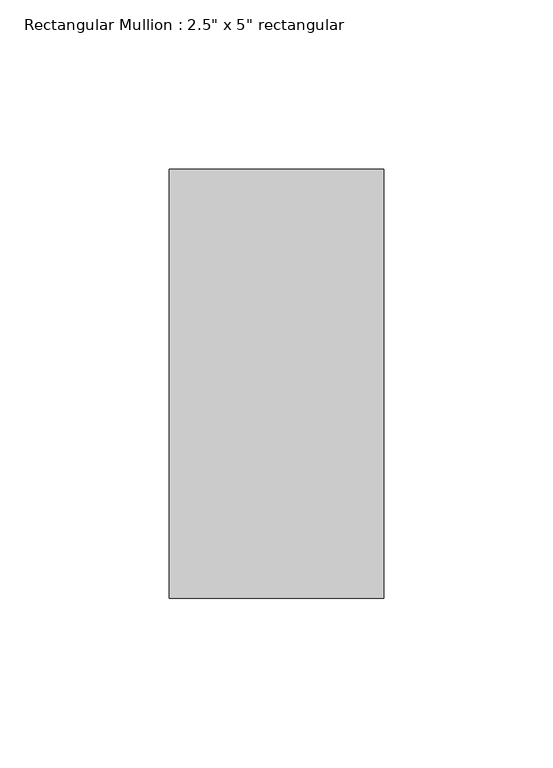
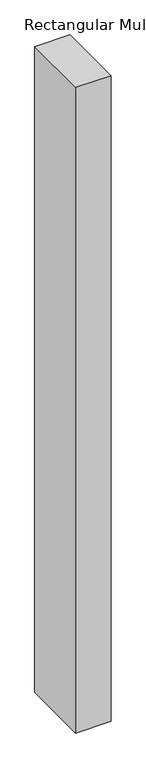
"""IFC4 building model written with IfcOpenShell, lengths in millimetres: member geometry."""

from ifc_helpers import new_model, si_unit, frame, origin, place, context, project, spatial, polyline, outline, extrude, source, transform, mapped, element, save


def member_d722639b(model_context):
    return source(origin(), model_context, "Body", "SweptSolid", [
        extrude(outline(polyline([(0.0, 63.5), (0.0, -63.5), (-63.5, -63.5), (-63.5, 63.5), (0.0, 63.5)])), frame((0.0, 0.0, -1224.7874211), z_axis=(0.0, 0.0, 1.0), x_axis=(1.0, 0.0, 0.0)), (0.0, 0.0, 1.0), 1224.7874211),
    ])


if __name__ == "__main__":
    model = new_model("IFC4")
    model_context = context("Model", 3, world=origin())
    ifc_project = project(units=[si_unit("LENGTHUNIT", "METRE", prefix="MILLI")], contexts=[model_context])
    site = spatial("IfcSite", under=ifc_project)
    building = spatial("IfcBuilding", under=site)
    placement = place(None, origin())
    member_shape = member_d722639b(model_context)
    element("IfcMember", 1, ObjectType="Rectangular Mullion : 2.5\" x 5\" rectangular", at=placement, inside=building, context=model_context, shape_type="MappedRepresentation", body=[
        mapped(member_shape, transform((0.0, 0.0, 0.0), x_axis=(1.0, 0.0, 0.0), y_axis=(0.0, 1.0, 0.0), z_axis=(0.0, 0.0, 1.0))),
    ])
    save(model, "model.ifc")

# Revit data of these elements
# Type "Rectangular Mullion : 2.5\" x 5\" rectangular"
#   built-in parameter 1007304 = 0.416667 (stored number, unit not read)
#   built-in parameter 1007301 = 0.104167 (stored number, unit not read)
#   built-in parameter 1007300 = 0.104167 (stored number, unit not read)
# Element 1 (IfcMember, "Rectangular Mullion : 2.5\" x 5\" rectangular")
#   Materials on its faces: "Aluminum"
# Materials
#   "Aluminum": class "Metal", colour RGB 247 247 247, transparency 0, Description = "Aluminum 6061", Cost = 0
